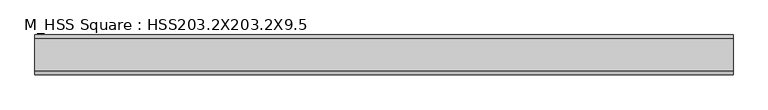
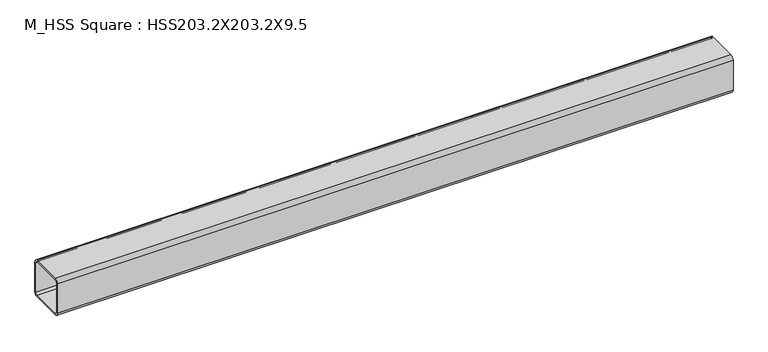
"""IFC4 building model written with IfcOpenShell, lengths in millimetres: member geometry, M_HSS Square : HSS203.2X203.2X9.5."""

from ifc_helpers import new_model, si_unit, point, frame, frame_2d, origin, place, context, project, spatial, polyline, circle_curve, trimmed, segment, composite_curve, outline, extrude, source, transform, mapped, element, save


def m_hss_square_hss203_2x203_2x9_5_07d005dd(model_context):
    return source(origin(), model_context, "Body", "SweptSolid", [
        extrude(outline(composite_curve([segment(trimmed(circle_curve(frame_2d((-82.44, 82.44)), 19.06), [point((-101.5, 82.44))], [point((-82.44, 101.5))], False, "CARTESIAN"), True, "CONTINUOUS"), segment(polyline([(-82.44, 101.5), (82.44, 101.5)]), True, "CONTINUOUS"), segment(trimmed(circle_curve(frame_2d((82.44, 82.44)), 19.06), [point((82.44, 101.5))], [point((101.5, 82.44))], False, "CARTESIAN"), True, "CONTINUOUS"), segment(polyline([(101.5, 82.44), (101.5, -82.44)]), True, "CONTINUOUS"), segment(trimmed(circle_curve(frame_2d((82.44, -82.44)), 19.06), [point((101.5, -82.44))], [point((82.44, -101.5))], False, "CARTESIAN"), True, "CONTINUOUS"), segment(polyline([(82.44, -101.5), (-82.44, -101.5)]), True, "CONTINUOUS"), segment(trimmed(circle_curve(frame_2d((-82.44, -82.44)), 19.06), [point((-82.44, -101.5))], [point((-101.5, -82.44))], False, "CARTESIAN"), True, "CONTINUOUS"), segment(polyline([(-101.5, -82.44), (-101.5, 82.44)]), True, "CONTINUOUS")], self_intersect=False), holes=[composite_curve([segment(polyline([(82.44, 91.97), (-82.44, 91.97)]), True, "CONTINUOUS"), segment(trimmed(circle_curve(frame_2d((-82.44, 82.44)), 9.53), [point((-82.44, 91.97))], [point((-91.97, 82.44))], True, "CARTESIAN"), True, "CONTINUOUS"), segment(polyline([(-91.97, 82.44), (-91.97, -82.44)]), True, "CONTINUOUS"), segment(trimmed(circle_curve(frame_2d((-82.44, -82.44)), 9.53), [point((-91.97, -82.44))], [point((-82.44, -91.97))], True, "CARTESIAN"), True, "CONTINUOUS"), segment(polyline([(-82.44, -91.97), (82.44, -91.97)]), True, "CONTINUOUS"), segment(trimmed(circle_curve(frame_2d((82.44, -82.44)), 9.53), [point((82.44, -91.97))], [point((91.97, -82.44))], True, "CARTESIAN"), True, "CONTINUOUS"), segment(polyline([(91.97, -82.44), (91.97, 82.44)]), True, "CONTINUOUS"), segment(trimmed(circle_curve(frame_2d((82.44, 82.44)), 9.53), [point((91.97, 82.44))], [point((82.44, 91.97))], True, "CARTESIAN"), True, "CONTINUOUS")], self_intersect=False)]), frame((-1777.2, 0.0, 0.0), z_axis=(1.0, 0.0, 0.0), x_axis=(0.0, 1.0, 0.0)), (0.0, 0.0, 1.0), 3554.4),
    ])


if __name__ == "__main__":
    model = new_model("IFC4")
    model_context = context("Model", 3, world=origin())
    ifc_project = project(units=[si_unit("LENGTHUNIT", "METRE", prefix="MILLI")], contexts=[model_context])
    site = spatial("IfcSite", under=ifc_project)
    building = spatial("IfcBuilding", under=site)
    placement = place(None, origin())
    m_hss_square_hss203_2x203_2x9_5_shape = m_hss_square_hss203_2x203_2x9_5_07d005dd(model_context)
    element("IfcMember", 1, ObjectType="M_HSS Square : HSS203.2X203.2X9.5", at=placement, inside=building, context=model_context, shape_type="MappedRepresentation", body=[
        mapped(m_hss_square_hss203_2x203_2x9_5_shape, transform((0.0, 0.0, 0.0), x_axis=(1.0, 0.0, 0.0), y_axis=(0.0, 1.0, 0.0), z_axis=(0.0, 0.0, 1.0))),
    ])
    save(model, "model.ifc")

# Revit data of these elements
# Type "M_HSS Square : HSS203.2X203.2X9.5"
#   Section Name Key = "HSS 8X8X3/8"
#   Width = 20.3 cm
#   Wall Nominal Thickness = 0.953 cm
#   Wall Design Thickness = 0.886 cm
#   Torsional Moment of Inertia = 6660.00 cm⁴
#   Torsional Modulus = 10930171.7 cm³
#   Section Area = 67.1 cm²
#   Plastic Modulus weak axis = 482.0 cm³
#   Plastic Modulus strong axis = 482.0 cm³
#   Outer Fillet = 1.906 cm
#   Nominal Weight = 55.9998 kgf/m
#   Moment of Inertia weak axis = 4160.00 cm⁴
#   Moment of Inertia strong axis = 4160.00 cm⁴
#   Length [instance default] = 1.524 m
#   Inner Fillet = 0.953 cm
#   Height = 20.3 cm
#   Elastic Modulus weak axis = 408.0 cm³
#   Elastic Modulus strong axis = 408.0 cm³
#   Centroid Vertical = 10.15 cm
#   Centroid Horizontal = 10.15 cm
#   Structural Material [instance default] = Steel, 45-345
# Element 1 (IfcMember, "M_HSS Square : HSS203.2X203.2X9.5")
#   Structural Material = Metal - Steel 43-275
#   Materials on its faces: "Metal - Steel 43-275"
# Materials
#   "Steel, 45-345": class "Metal", colour RGB 247 247 247, transparency 0, Description = "Steel 345 MPa", Cost = 0
#   "Metal - Steel 43-275": class "Metal", colour RGB 247 247 247, transparency 0, Cost = 0
